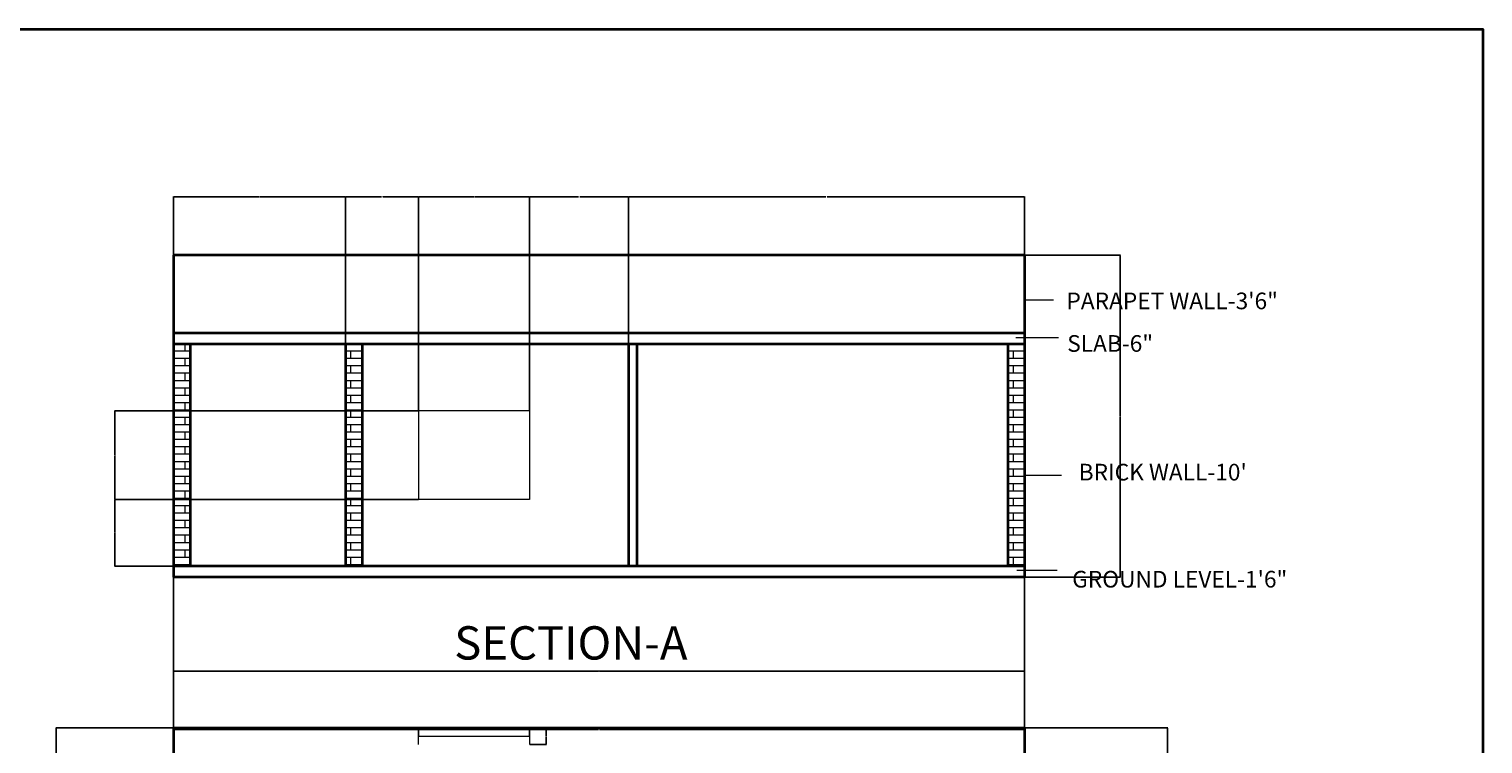
# Model space of a CAD drawing. Units: inches. Extents: x 1152 to 2588, y 1459 to 2618.
# Tile 17 of 17: x 1802 to 2588, y 2231 to 2618. Entities that reach past the tile are written whole.
import ezdxf

# ---------------------------------------------------------------- set-up
doc = ezdxf.new("R2010")
doc.units = ezdxf.units.IN
for name, color, linetype, lineweight in [('A-ANNO-DIMS', 2, 'Continuous', 18), ('A-ANNO-SYMB', 3, 'Continuous', 18), ('A-ANNO-TEXT', 7, 'Continuous', 18), ('A-ANNO-TTLB', 7, 'Continuous', 35), ('A-GLAZ', 4, 'Continuous', 18), ('A-SECT', 7, 'Continuous', 35), ('A-WALL', 7, 'Continuous', 35), ('A-WALL-PATT', 8, 'Continuous', 13)]:
    doc.layers.add(name, color=color, linetype=linetype, lineweight=lineweight)
doc.styles.get("Standard").update_dxf_attribs({"font": 'arial.ttf'})
doc.dimstyles.get("Standard").update_dxf_attribs({"dimtxt": 0.18, "dimasz": 0.18, "dimexe": 0.18, "dimexo": 0.0625, "dimgap": 0.09, "dimtad": 0, "dimtih": 1, "dimtoh": 1, "dimdec": 4, "dimzin": 0, "dimdsep": 46, "dimtxsty": 'Standard', "dimcen": 0.09, "dimadec": 0, "dimazin": 0, "dimtfac": 1, "dimtdec": 4, "dimtofl": 0, "dimtmove": 0, "dimatfit": 3, "dimfxl": 1, "dimtolj": 1, "dimtzin": 0, "dimarcsym": 0})

# ---------------------------------------------------------------- blocks, each defined once
blk = doc.blocks.new('WIN-60-BED-NORTH')
for p, q in [((0, 0), (0, 9)), ((0, 9), (0, 4.5)), ((60, 4.5), (60, 9)), ((60, 9), (60, 0)), ((0, 4.5), (60, 4.5))]:
    blk.add_line(p, q)
blk = doc.blocks.new('*D65')
at = {"layer": 'A-ANNO-DIMS', "color": 0, "lineweight": -2, "transparency": 16777216}
for p, q in [((2072.46, 2240.05), (2081.57, 2240.05)), ((2081.39, 2239.87), (2081.39, 2235.73)), ((2081.39, 2231.23), (2081.39, 2235.36)), ((2072.46, 2231.05), (2081.57, 2231.05))]:
    blk.add_line(p, q, dxfattribs=at)
at = {"layer": 'A-ANNO-DIMS', "color": 0, "transparency": 16777216}
for points in [[(2081.36, 2239.87), (2081.42, 2239.87), (2081.39, 2240.05)], [(2081.36, 2231.23), (2081.42, 2231.23), (2081.39, 2231.05)]]:
    blk.add_solid(points, dxfattribs=at)
at = {"layer": 'Defpoints', "color": 0, "transparency": 16777216}
for p in [(2072.39, 2240.05), (2081.39, 2240.05), (2072.39, 2231.05)]:
    blk.add_point(p, dxfattribs=at)
at = {"layer": 'A-ANNO-DIMS', "color": 0, "transparency": 16777216, "insert": (2081.39, 2235.55), "char_height": 0.18, "attachment_point": 5}
blk.add_mtext('\\A1;9 TYP.', dxfattribs=at)
blk = doc.blocks.new('*D77')
at = {"layer": 'A-ANNO-DIMS', "color": 0, "lineweight": -2, "transparency": 16777216}
for p, q in [((1879.88, 2240.11), (1879.88, 2270.83)), ((1880.06, 2270.65), (2109.59, 2270.65)), ((2339.7, 2270.65), (2110.18, 2270.65)), ((2339.88, 2240.11), (2339.88, 2270.83))]:
    blk.add_line(p, q, dxfattribs=at)
at = {"layer": 'A-ANNO-DIMS', "color": 0, "transparency": 16777216}
for points in [[(1880.06, 2270.68), (1880.06, 2270.62), (1879.88, 2270.65)], [(2339.7, 2270.68), (2339.7, 2270.62), (2339.88, 2270.65)]]:
    blk.add_solid(points, dxfattribs=at)
at = {"layer": 'Defpoints', "color": 0, "transparency": 16777216}
for p in [(2339.88, 2270.65), (1879.88, 2240.05), (2339.88, 2240.05)]:
    blk.add_point(p, dxfattribs=at)
at = {"layer": 'A-ANNO-DIMS', "color": 0, "transparency": 16777216, "insert": (2109.88, 2270.65), "char_height": 0.18, "attachment_point": 5}
blk.add_mtext('\\A1;460', dxfattribs=at)
blk = doc.blocks.new('*D78')
at = {"layer": 'A-ANNO-DIMS', "color": 0, "lineweight": -2, "transparency": 16777216}
for p, q in [((2339.95, 2240.05), (2417.36, 2240.05)), ((2417.18, 2239.87), (2417.18, 1937.73)), ((2417.18, 1635.23), (2417.18, 1937.36)), ((2339.95, 1635.05), (2417.36, 1635.05))]:
    blk.add_line(p, q, dxfattribs=at)
at = {"layer": 'A-ANNO-DIMS', "color": 0, "transparency": 16777216}
for points in [[(2417.15, 2239.87), (2417.21, 2239.87), (2417.18, 2240.05)], [(2417.15, 1635.23), (2417.21, 1635.23), (2417.18, 1635.05)]]:
    blk.add_solid(points, dxfattribs=at)
at = {"layer": 'Defpoints', "color": 0, "transparency": 16777216}
for p in [(2339.88, 2240.05), (2417.18, 2240.05), (2339.88, 1635.05)]:
    blk.add_point(p, dxfattribs=at)
at = {"layer": 'A-ANNO-DIMS', "color": 0, "transparency": 16777216, "insert": (2417.18, 1937.55), "char_height": 0.18, "attachment_point": 5}
blk.add_mtext('\\A1;605', dxfattribs=at)
blk = doc.blocks.new('*D84')
at = {"layer": 'A-ANNO-DIMS', "color": 0, "lineweight": -2, "transparency": 16777216}
for p, q in [((1879.82, 2240.05), (1816.39, 2240.05)), ((1816.57, 2239.87), (1816.57, 2216.58)), ((1816.57, 2192.93), (1816.57, 2216.22)), ((1879.82, 2192.75), (1816.39, 2192.75))]:
    blk.add_line(p, q, dxfattribs=at)
at = {"layer": 'A-ANNO-DIMS', "color": 0, "transparency": 16777216}
for points in [[(1816.54, 2239.87), (1816.6, 2239.87), (1816.57, 2240.05)], [(1816.54, 2192.93), (1816.6, 2192.93), (1816.57, 2192.75)]]:
    blk.add_solid(points, dxfattribs=at)
at = {"layer": 'Defpoints', "color": 0, "transparency": 16777216}
for p in [(1816.57, 2240.05), (1879.88, 2240.05), (1879.88, 2192.75)]:
    blk.add_point(p, dxfattribs=at)
at = {"layer": 'A-ANNO-DIMS', "color": 0, "transparency": 16777216, "insert": (1816.57, 2216.4), "char_height": 0.18, "attachment_point": 5}
blk.add_mtext('\\A1;47.3', dxfattribs=at)
blk = doc.blocks.new('*D99')
at = {"layer": 'A-ANNO-DIMS', "color": 0, "lineweight": -2, "transparency": 16777216}
for p, q in [((1879.88, 2321.33), (1879.88, 2238.88)), ((2339.88, 2321.33), (2339.88, 2238.88)), ((1880.06, 2239.06), (2109.59, 2239.06)), ((2339.7, 2239.06), (2110.18, 2239.06))]:
    blk.add_line(p, q, dxfattribs=at)
at = {"layer": 'A-ANNO-DIMS', "color": 0, "transparency": 16777216}
for points in [[(1880.06, 2239.09), (1880.06, 2239.03), (1879.88, 2239.06)], [(2339.7, 2239.09), (2339.7, 2239.03), (2339.88, 2239.06)]]:
    blk.add_solid(points, dxfattribs=at)
at = {"layer": 'Defpoints', "color": 0, "transparency": 16777216}
for p in [(1879.88, 2321.39), (2339.88, 2321.39), (2339.88, 2239.06)]:
    blk.add_point(p, dxfattribs=at)
at = {"layer": 'A-ANNO-DIMS', "color": 0, "transparency": 16777216, "insert": (2109.88, 2239.06), "char_height": 0.18, "attachment_point": 5}
blk.add_mtext('\\A1;460', dxfattribs=at)
blk = doc.blocks.new('*D100')
at = {"layer": 'A-ANNO-DIMS', "color": 0, "lineweight": -2, "transparency": 16777216}
for p, q in [((2339.95, 2495.39), (2391.77, 2495.39)), ((2391.59, 2495.21), (2391.59, 2408.57)), ((2391.59, 2321.57), (2391.59, 2408.21)), ((2339.95, 2321.39), (2391.77, 2321.39))]:
    blk.add_line(p, q, dxfattribs=at)
at = {"layer": 'A-ANNO-DIMS', "color": 0, "transparency": 16777216}
for points in [[(2391.56, 2495.21), (2391.62, 2495.21), (2391.59, 2495.39)], [(2391.56, 2321.57), (2391.62, 2321.57), (2391.59, 2321.39)]]:
    blk.add_solid(points, dxfattribs=at)
at = {"layer": 'Defpoints', "color": 0, "transparency": 16777216}
for p in [(2339.88, 2495.39), (2391.59, 2495.39), (2339.88, 2321.39)]:
    blk.add_point(p, dxfattribs=at)
at = {"layer": 'A-ANNO-DIMS', "color": 0, "transparency": 16777216, "insert": (2391.59, 2408.39), "char_height": 0.18, "attachment_point": 5}
blk.add_mtext('\\A1;174', dxfattribs=at)
blk = doc.blocks.new('*D101')
at = {"layer": 'A-ANNO-DIMS', "color": 0, "lineweight": -2, "transparency": 16777216}
for p, q in [((1879.88, 2495.45), (1879.88, 2527.17)), ((1880.06, 2526.99), (1926.17, 2526.99)), ((1972.7, 2526.99), (1926.6, 2526.99)), ((1972.88, 2447.45), (1972.88, 2527.17))]:
    blk.add_line(p, q, dxfattribs=at)
at = {"layer": 'A-ANNO-DIMS', "color": 0, "transparency": 16777216}
for points in [[(1880.06, 2527.02), (1880.06, 2526.96), (1879.88, 2526.99)], [(1972.7, 2527.02), (1972.7, 2526.96), (1972.88, 2526.99)]]:
    blk.add_solid(points, dxfattribs=at)
at = {"layer": 'Defpoints', "color": 0, "transparency": 16777216}
for p in [(1972.88, 2526.99), (1879.88, 2495.39), (1972.88, 2447.39)]:
    blk.add_point(p, dxfattribs=at)
at = {"layer": 'A-ANNO-DIMS', "color": 0, "transparency": 16777216, "insert": (1926.38, 2526.99), "char_height": 0.18, "attachment_point": 5}
blk.add_mtext('\\A1;93', dxfattribs=at)
blk = doc.blocks.new('*D102')
at = {"layer": 'A-ANNO-DIMS', "color": 0, "lineweight": -2, "transparency": 16777216}
for p, q in [((1972.88, 2447.45), (1972.88, 2527.17)), ((1973.06, 2526.99), (1992.26, 2526.99)), ((2012.21, 2526.99), (1993.02, 2526.99)), ((2012.39, 2411.45), (2012.39, 2527.17))]:
    blk.add_line(p, q, dxfattribs=at)
at = {"layer": 'A-ANNO-DIMS', "color": 0, "transparency": 16777216}
for points in [[(1973.06, 2527.02), (1973.06, 2526.96), (1972.88, 2526.99)], [(2012.21, 2527.02), (2012.21, 2526.96), (2012.39, 2526.99)]]:
    blk.add_solid(points, dxfattribs=at)
at = {"layer": 'Defpoints', "color": 0, "transparency": 16777216}
for p in [(2012.39, 2526.99), (1972.88, 2447.39), (2012.39, 2411.39)]:
    blk.add_point(p, dxfattribs=at)
at = {"layer": 'A-ANNO-DIMS', "color": 0, "transparency": 16777216, "insert": (1992.64, 2526.99), "char_height": 0.18, "attachment_point": 5}
blk.add_mtext('\\A1;39.51', dxfattribs=at)
blk = doc.blocks.new('*D103')
at = {"layer": 'A-ANNO-DIMS', "color": 0, "lineweight": -2, "transparency": 16777216}
for p, q in [((2012.39, 2411.45), (2012.39, 2527.17)), ((2012.57, 2526.99), (2042.18, 2526.99)), ((2072.21, 2526.99), (2042.61, 2526.99)), ((2072.39, 2411.45), (2072.39, 2527.17))]:
    blk.add_line(p, q, dxfattribs=at)
at = {"layer": 'A-ANNO-DIMS', "color": 0, "transparency": 16777216}
for points in [[(2012.57, 2527.02), (2012.57, 2526.96), (2012.39, 2526.99)], [(2072.21, 2527.02), (2072.21, 2526.96), (2072.39, 2526.99)]]:
    blk.add_solid(points, dxfattribs=at)
at = {"layer": 'Defpoints', "color": 0, "transparency": 16777216}
for p in [(2072.39, 2526.99), (2012.39, 2411.39), (2072.39, 2411.39)]:
    blk.add_point(p, dxfattribs=at)
at = {"layer": 'A-ANNO-DIMS', "color": 0, "transparency": 16777216, "insert": (2042.39, 2526.99), "char_height": 0.18, "attachment_point": 5}
blk.add_mtext('\\A1;60', dxfattribs=at)
blk = doc.blocks.new('*D104')
at = {"layer": 'A-ANNO-DIMS', "color": 0, "lineweight": -2, "transparency": 16777216}
for p, q in [((2072.39, 2411.45), (2072.39, 2527.17)), ((2072.57, 2526.99), (2098.75, 2526.99)), ((2125.7, 2526.99), (2099.53, 2526.99)), ((2125.88, 2447.45), (2125.88, 2527.17))]:
    blk.add_line(p, q, dxfattribs=at)
at = {"layer": 'A-ANNO-DIMS', "color": 0, "transparency": 16777216}
for points in [[(2072.57, 2527.02), (2072.57, 2526.96), (2072.39, 2526.99)], [(2125.7, 2527.02), (2125.7, 2526.96), (2125.88, 2526.99)]]:
    blk.add_solid(points, dxfattribs=at)
at = {"layer": 'Defpoints', "color": 0, "transparency": 16777216}
for p in [(2125.88, 2526.99), (2125.88, 2447.39), (2072.39, 2411.39)]:
    blk.add_point(p, dxfattribs=at)
at = {"layer": 'A-ANNO-DIMS', "color": 0, "transparency": 16777216, "insert": (2099.14, 2526.99), "char_height": 0.18, "attachment_point": 5}
blk.add_mtext('\\A1;53.49', dxfattribs=at)
blk = doc.blocks.new('*D105')
at = {"layer": 'A-ANNO-DIMS', "color": 0, "lineweight": -2, "transparency": 16777216}
for p, q in [((2125.88, 2447.45), (2125.88, 2527.17)), ((2126.06, 2526.99), (2232.59, 2526.99)), ((2339.7, 2526.99), (2233.17, 2526.99)), ((2339.88, 2495.45), (2339.88, 2527.17))]:
    blk.add_line(p, q, dxfattribs=at)
at = {"layer": 'A-ANNO-DIMS', "color": 0, "transparency": 16777216}
for points in [[(2126.06, 2527.02), (2126.06, 2526.96), (2125.88, 2526.99)], [(2339.7, 2527.02), (2339.7, 2526.96), (2339.88, 2526.99)]]:
    blk.add_solid(points, dxfattribs=at)
at = {"layer": 'Defpoints', "color": 0, "transparency": 16777216}
for p in [(2339.88, 2526.99), (2339.88, 2495.39), (2125.88, 2447.39)]:
    blk.add_point(p, dxfattribs=at)
at = {"layer": 'A-ANNO-DIMS', "color": 0, "transparency": 16777216, "insert": (2232.88, 2526.99), "char_height": 0.18, "attachment_point": 5}
blk.add_mtext('\\A1;214', dxfattribs=at)
blk = doc.blocks.new('*D106')
at = {"layer": 'A-ANNO-DIMS', "color": 0, "lineweight": -2, "transparency": 16777216}
for p, q in [((2012.33, 2363.39), (1848.1, 2363.39)), ((1848.28, 2363.21), (1848.28, 2345.57)), ((1848.28, 2327.57), (1848.28, 2345.21)), ((1888.82, 2327.39), (1848.1, 2327.39))]:
    blk.add_line(p, q, dxfattribs=at)
at = {"layer": 'A-ANNO-DIMS', "color": 0, "transparency": 16777216}
for points in [[(1848.25, 2363.21), (1848.31, 2363.21), (1848.28, 2363.39)], [(1848.25, 2327.57), (1848.31, 2327.57), (1848.28, 2327.39)]]:
    blk.add_solid(points, dxfattribs=at)
at = {"layer": 'Defpoints', "color": 0, "transparency": 16777216}
for p in [(2012.39, 2363.39), (1848.28, 2327.39), (1888.88, 2327.39)]:
    blk.add_point(p, dxfattribs=at)
at = {"layer": 'A-ANNO-DIMS', "color": 0, "transparency": 16777216, "insert": (1848.28, 2345.39), "char_height": 0.18, "attachment_point": 5}
blk.add_mtext('\\A1;36', dxfattribs=at)
blk = doc.blocks.new('*D107')
at = {"layer": 'A-ANNO-DIMS', "color": 0, "lineweight": -2, "transparency": 16777216}
for p, q in [((2012.33, 2411.39), (1848.1, 2411.39)), ((1848.28, 2411.21), (1848.28, 2387.57)), ((1848.28, 2363.57), (1848.28, 2387.21)), ((2012.33, 2363.39), (1848.1, 2363.39))]:
    blk.add_line(p, q, dxfattribs=at)
at = {"layer": 'A-ANNO-DIMS', "color": 0, "transparency": 16777216}
for points in [[(1848.25, 2411.21), (1848.31, 2411.21), (1848.28, 2411.39)], [(1848.25, 2363.57), (1848.31, 2363.57), (1848.28, 2363.39)]]:
    blk.add_solid(points, dxfattribs=at)
at = {"layer": 'Defpoints', "color": 0, "transparency": 16777216}
for p in [(2012.39, 2411.39), (1848.28, 2363.39), (2012.39, 2363.39)]:
    blk.add_point(p, dxfattribs=at)
at = {"layer": 'A-ANNO-DIMS', "color": 0, "transparency": 16777216, "insert": (1848.28, 2387.39), "char_height": 0.18, "attachment_point": 5}
blk.add_mtext('\\A1;48', dxfattribs=at)

msp = doc.modelspace()

# ---------------------------------------------------------------- hatches: boundary and pattern name
at = {"layer": 'A-WALL-PATT'}
h = msp.add_hatch(dxfattribs=at)
h.set_pattern_fill('AR-BRSTD', color=256, scale=0.0587525, style=0)
h.paths.add_polyline_path([(1879.8841, 2327.3911), (1888.8841, 2327.3911), (1888.8841, 2447.3911), (1879.8841, 2447.3911)])
h = msp.add_hatch(dxfattribs=at)
h.set_pattern_fill('AR-BRSTD', color=256, scale=0.0587525, style=0)
h.paths.add_polyline_path([(1972.8841, 2327.3911), (1981.8841, 2327.3911), (1981.8841, 2447.3911), (1972.8841, 2447.3911)])
h = msp.add_hatch(dxfattribs=at)
h.set_pattern_fill('AR-BRSTD', color=256, scale=0.0587525, style=0)
h.paths.add_polyline_path([(2330.8841, 2327.3911), (2339.8841, 2327.3911), (2339.8841, 2447.3911), (2330.8841, 2447.3911)])

# ---------------------------------------------------------------- linework, layer by layer
at = {"layer": 'A-ANNO-SYMB'}
for p, q in [((2339.8841, 2471.269), (2355.6424, 2471.269)), ((2335.1606, 2450.932), (2358.2739, 2450.932)), ((2339.8841, 2376.5143), (2359.9916, 2376.5143)), ((2335.6952, 2325.1435), (2357.5553, 2325.1435))]:
    msp.add_line(p, q, dxfattribs=at)
at = {"layer": 'A-ANNO-TEXT'}
msp.add_line((2176.5134, 2270.6581), (2027.0934, 2270.6581), dxfattribs=at)
at = {"layer": 'A-ANNO-TTLB'}
msp.add_lwpolyline([(1152.3215, 2617.6685), (2587.6987, 2617.6685), (2587.6987, 1459.3148), (1152.3215, 1459.3148)], close=True, dxfattribs=at)
at = {"layer": 'A-GLAZ'}
for p, q in [((2012.3947, 2411.3911), (2012.3947, 2363.3911)), ((2072.3947, 2411.3911), (2012.3947, 2411.3911)), ((2072.3947, 2411.3911), (2072.3947, 2363.3911)), ((2072.3947, 2363.3911), (2012.3947, 2363.3911))]:
    msp.add_line(p, q, dxfattribs=at)
at = {"layer": 'A-SECT'}
for p, q in [((1879.8841, 2495.3911), (1879.8841, 2321.3911)), ((2339.8841, 2495.3911), (1879.8841, 2495.3911)), ((2339.8841, 2495.3911), (2339.8841, 2321.3911)), ((2339.8841, 2453.3911), (1879.8841, 2453.3911)), ((2339.8841, 2447.3911), (1879.8841, 2447.3911)), ((1888.8841, 2447.3911), (1888.8841, 2327.3911)), ((1972.8841, 2447.3911), (1972.8841, 2327.3911)), ((1981.8841, 2447.3911), (1981.8841, 2327.3911)), ((2125.8841, 2447.3911), (2125.8841, 2327.3911)), ((2130.3841, 2447.3911), (2130.3841, 2327.3911)), ((2330.8841, 2447.3911), (2330.8841, 2327.3911)), ((2339.8841, 2327.3911), (1879.8841, 2327.3911)), ((2339.8841, 2321.3911), (1879.8841, 2321.3911))]:
    msp.add_line(p, q, dxfattribs=at)
at = {"layer": 'A-WALL'}
for p, q in [((1879.8841, 2240.0458), (2339.8841, 2240.0458)), ((1879.8841, 2240.0458), (1879.8841, 2084.0458)), ((2339.8841, 2240.0458), (2339.8841, 1635.0458))]:
    msp.add_line(p, q, dxfattribs=at)

# ---------------------------------------------------------------- block references
at = {"layer": 'A-GLAZ'}
msp.add_blockref('WIN-60-BED-NORTH', (2012.3946, 2231.046), dxfattribs=at)

# ---------------------------------------------------------------- texts
at = {"layer": 'A-ANNO-TEXT', "attachment_point": 1}
for s, width, insert, char_height in [('PARAPET WALL-3\'6"', 465.245579, (2362.5748, 2475.2394), 9), ('SLAB-6"', 41.254405, (2362.9971, 2452.239), 9), ("BRICK WALL-10'", 182.878759, (2369.189, 2382.6907), 9), ('GROUND LEVEL-1\'6"', 165.246053, (2365.6772, 2324.8236), 9), ('\\pxt3;SECTION-A', 342.568341, (2031.6352, 2294.8975), 18)]:
    msp.add_mtext_dynamic_manual_height_columns(s, width=width, gutter_width=12.5, heights=[0], dxfattribs=dict(at, insert=insert, char_height=char_height))

# ---------------------------------------------------------------- dimensions: what is measured, and where the dimension line sits
at = {"layer": 'A-ANNO-DIMS'}
for base, p1, p2, override, picture, middle in [((1972.8841, 2526.9911), (1879.8841, 2495.3911), (1972.8841, 2447.3911), {"dimdec": 0, "dimlfac": 1, "dimrnd": 0, "dimzin": 0, "dimdsep": 46, "dimlunit": 2}, '*D101', (1926.3841, 2526.9911)), ((2012.3947, 2526.9911), (1972.8841, 2447.3911), (2012.3947, 2411.3911), {"dimdec": 2, "dimlfac": 1, "dimrnd": 0, "dimzin": 0, "dimdsep": 46, "dimlunit": 2}, '*D102', (1992.6394, 2526.9911)), ((2072.3947, 2526.9911), (2012.3947, 2411.3911), (2072.3947, 2411.3911), {"dimdec": 0, "dimlfac": 1, "dimrnd": 0, "dimzin": 0, "dimdsep": 46, "dimlunit": 2}, '*D103', (2042.3947, 2526.9911)), ((2125.8841, 2526.9911), (2072.3947, 2411.3911), (2125.8841, 2447.3911), {"dimdec": 2, "dimlfac": 1, "dimrnd": 0, "dimzin": 0, "dimdsep": 46, "dimlunit": 2}, '*D104', (2099.1394, 2526.9911)), ((2339.8841, 2526.9911), (2125.8841, 2447.3911), (2339.8841, 2495.3911), {"dimdec": 0, "dimlfac": 1, "dimrnd": 0, "dimzin": 0, "dimdsep": 46, "dimlunit": 2}, '*D105', (2232.8841, 2526.9911)), ((2339.8841, 2239.0581), (1879.8841, 2321.3911), (2339.8841, 2321.3911), {"dimdec": 0, "dimlfac": 1, "dimrnd": 0, "dimzin": 0, "dimdsep": 46, "dimlunit": 2}, '*D99', (2109.8841, 2239.0581)), ((2339.8841, 2270.6458), (1879.8841, 2240.0458), (2339.8841, 2240.0458), {"dimdec": 0, "dimlfac": 1, "dimrnd": 0, "dimzin": 0, "dimdsep": 46, "dimlunit": 2}, '*D77', (2109.8841, 2270.6458))]:
    dim = msp.add_linear_dim(base=base, p1=p1, p2=p2, dimstyle='Standard', override=override, dxfattribs=at)
    dim.commit()
    dim.dimension.update_dxf_attribs({"geometry": picture, "text_midpoint": middle})
for base, p1, p2, override, picture, middle in [((2391.5916, 2495.3911), (2339.8841, 2321.3911), (2339.8841, 2495.3911), {"dimdec": 0, "dimlfac": 1, "dimrnd": 0, "dimzin": 0, "dimdsep": 46, "dimlunit": 2}, '*D100', (2391.5916, 2408.3911)), ((1848.2841, 2363.3911), (2012.3947, 2411.3911), (2012.3947, 2363.3911), {"dimdec": 0, "dimlfac": 1, "dimrnd": 0, "dimzin": 0, "dimdsep": 46, "dimlunit": 2}, '*D107', (1848.2841, 2387.3911)), ((1848.2841, 2327.3911), (2012.3947, 2363.3911), (1888.8841, 2327.3911), {"dimdec": 0, "dimlfac": 1, "dimrnd": 0, "dimzin": 0, "dimdsep": 46, "dimlunit": 2}, '*D106', (1848.2841, 2345.3911)), ((1816.569, 2240.0458), (1879.8841, 2192.7491), (1879.8841, 2240.0458), {"dimdec": 1, "dimlfac": 1, "dimrnd": 0, "dimzin": 0, "dimdsep": 46, "dimlunit": 2}, '*D84', (1816.569, 2216.3975)), ((2417.1775, 2240.0458), (2339.8841, 1635.0458), (2339.8841, 2240.0458), {"dimdec": 0, "dimlfac": 1, "dimrnd": 0, "dimzin": 0, "dimdsep": 46, "dimlunit": 2}, '*D78', (2417.1775, 1937.5458))]:
    dim = msp.add_linear_dim(base=base, p1=p1, p2=p2, angle=90, dimstyle='Standard', override=override, dxfattribs=at)
    dim.commit()
    dim.dimension.update_dxf_attribs({"geometry": picture, "text_midpoint": middle})
dim = msp.add_linear_dim(base=(2081.3947, 2240.0458), p1=(2072.3947, 2231.0458), p2=(2072.3947, 2240.0458), angle=90, text='<> TYP.', dimstyle='Standard', override={"dimdec": 0, "dimlfac": 1, "dimrnd": 0, "dimzin": 0, "dimdsep": 46, "dimlunit": 2}, dxfattribs=at)
dim.commit()
dim.dimension.update_dxf_attribs({"geometry": '*D65', "text_midpoint": (2081.3947, 2235.5458)})

doc.saveas('drawing.dxf')
